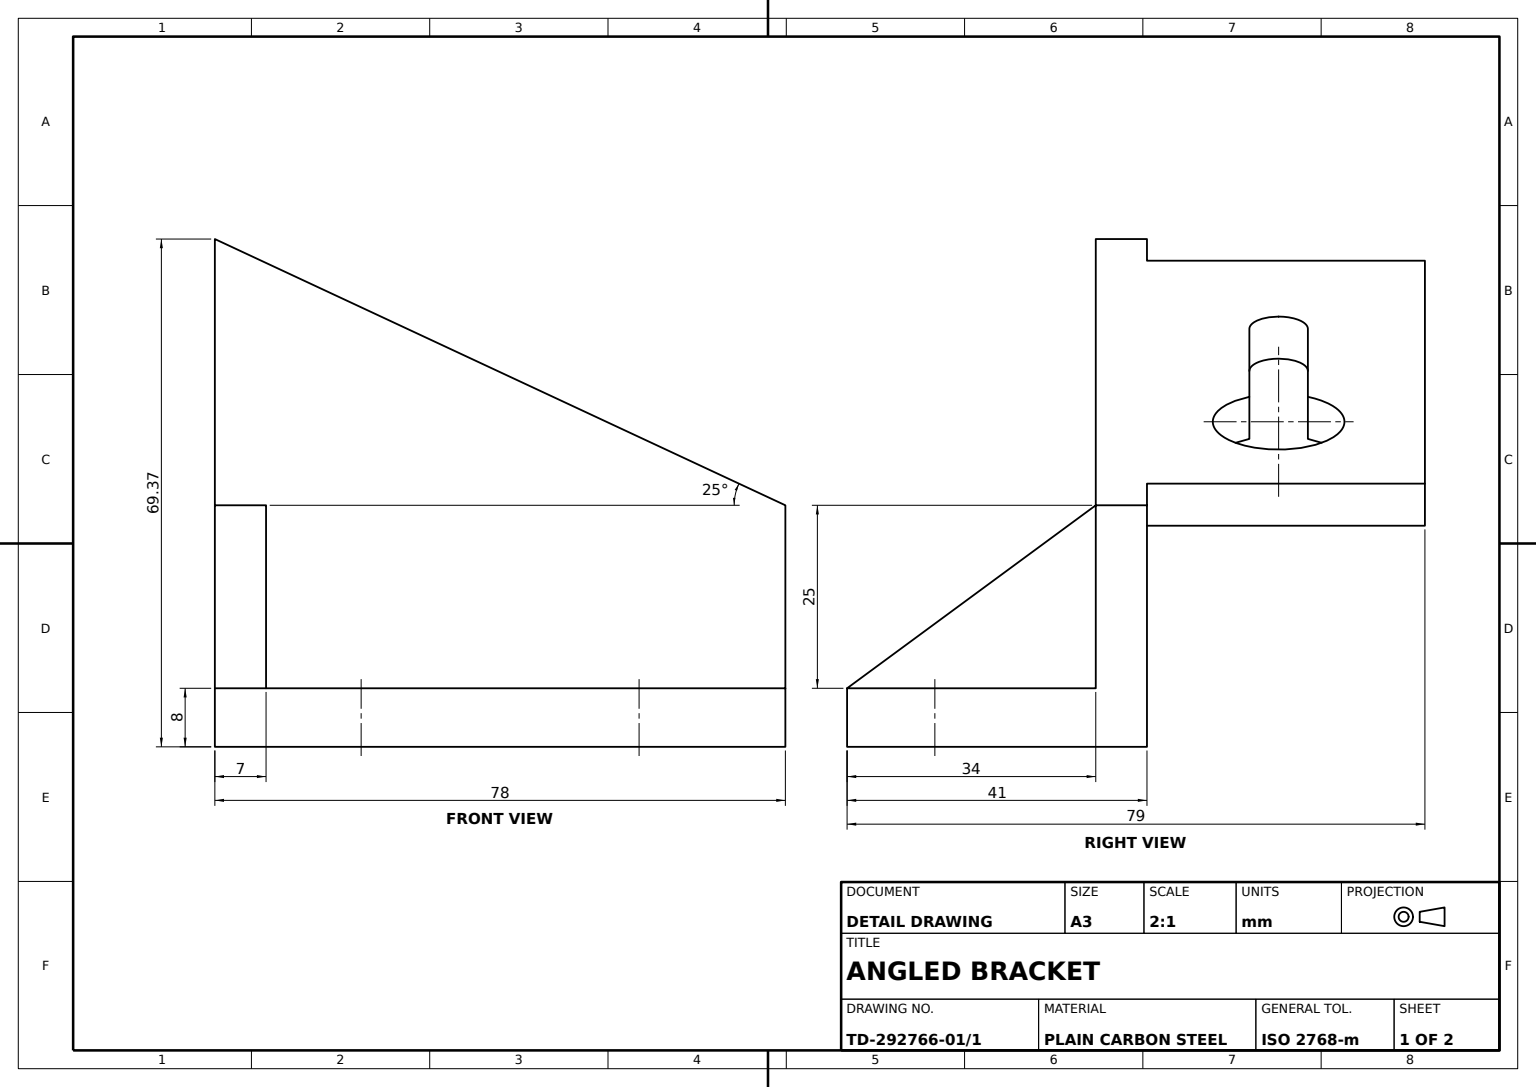
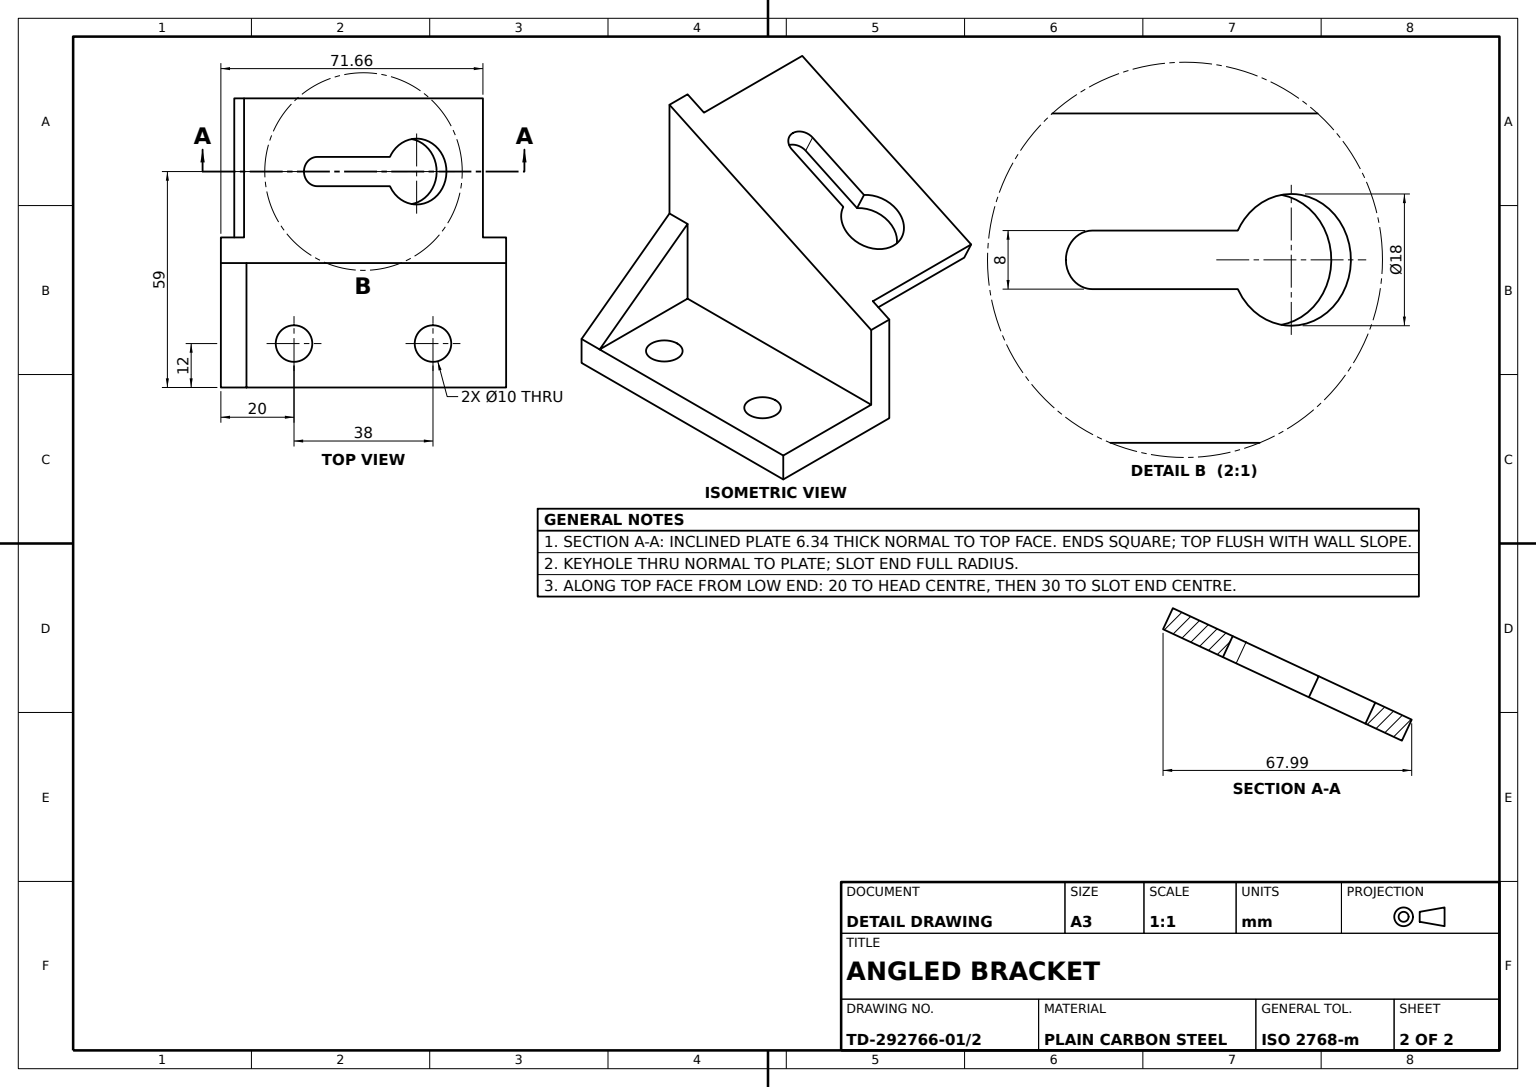
from build123d import *

# Parameters (mm, degrees)
BASE_PLATE_SKETCH_W                  = 78
BASE_PLATE_SKETCH_H                  = 41
BASE_PLATE_SKETCH_R                  = 5
BASE_PLATE_WITH_MOUNTING_HOLES_DEPTH = 8
UPRIGHT_WALL_SKETCH_W                = 7
UPRIGHT_WALL_SKETCH_H                = 41
UPRIGHT_WALL_DEPTH                   = 38
BACK_PLATE_SKETCH_W                  = 78
BACK_PLATE_SKETCH_H                  = 7
BACK_PLATE_DEPTH                     = 82
WALL_TRIM_CUT_DEPTH                  = 58
ANGLED_TRIM_CUT_25DEG_DEPTH          = 58
INCLINED_FLANGE_DEPTH                = 38
FLANGE_PROFILE_CUT_SKETCH_W          = 9.958327832
FLANGE_PROFILE_CUT_SKETCH_H          = 38
FLANGE_PROFILE_CUT_SKETCH_W_2        = 7
FLANGE_PROFILE_CUT_DEPTH             = 38
KEYHOLE_SLOT_DIA18_X_W8_REACH        = 92.402


with BuildPart() as part:
    # Base Plate Sketch → Base Plate with Mounting Holes (new body)
    with BuildSketch(Plane(origin=(0, 0, 0), x_dir=(1, 0, 0), z_dir=(0, 1, 0))):
        with Locations((0, -4)):
            Rectangle(BASE_PLATE_SKETCH_W, BASE_PLATE_SKETCH_H)
        with Locations(Location((-19, -12.5, 0), (0, 0, 270))):
            Circle(BASE_PLATE_SKETCH_R, mode=Mode.SUBTRACT)
        with Locations(Location((19, -12.5, 0), (0, 0, 270))):
            Circle(BASE_PLATE_SKETCH_R, mode=Mode.SUBTRACT)
    extrude(amount=BASE_PLATE_WITH_MOUNTING_HOLES_DEPTH)

    # Upright Wall Sketch → Upright Wall (add)
    with BuildSketch(Plane(origin=(0, 8, 0), x_dir=(1, 0, 0), z_dir=(0, 1, 0))):
        with Locations((-35.5, -4)):
            Rectangle(UPRIGHT_WALL_SKETCH_W, UPRIGHT_WALL_SKETCH_H)
    extrude(amount=UPRIGHT_WALL_DEPTH)

    # Back Plate Sketch → Back Plate (add)
    with BuildSketch(Plane(origin=(0, 8, 0), x_dir=(1, 0, 0), z_dir=(0, 1, 0))):
        with Locations((0, 13)):
            Rectangle(BACK_PLATE_SKETCH_W, BACK_PLATE_SKETCH_H)
    extrude(amount=BACK_PLATE_DEPTH)

    # Wall Trim Sketch → Wall Trim Cut (cut)
    with BuildSketch(Plane(origin=(-32, 0, 0), x_dir=(0, 0, -1), z_dir=(1, 0, 0))):
        Polygon((9.5, 33), (-24.5, 8), (-24.5, 46), (9.5, 46), align=None)
    extrude(amount=-WALL_TRIM_CUT_DEPTH, mode=Mode.SUBTRACT)

    # Angled Trim Sketch 25deg → Angled Trim Cut 25deg (cut)
    with BuildSketch(Plane.XY.offset(-9.5)):
        Polygon((-39, 69.371997336), (39, 33), (39, 90), (-39, 90), align=None)
    extrude(amount=-ANGLED_TRIM_CUT_25DEG_DEPTH, mode=Mode.SUBTRACT)

    # Inclined Flange Sketch → Inclined Flange (add)
    with BuildSketch(Plane(origin=(0, 0, -16.5), x_dir=(-1, 0, 0), z_dir=(0, 0, -1))):
        Polygon((-39, 33), (39, 69.371997336), (39, 62.371997336), (-39, 26), align=None)
    extrude(amount=INCLINED_FLANGE_DEPTH)

    # Flange Profile Cut Sketch → Flange Profile Cut (cut)
    with BuildSketch(Plane(origin=(19.605374923, 42.043862201, 0), x_dir=(0.9063077870366495, -0.42261826174070033, 0), z_dir=(0.42261826174070033, 0.9063077870366495, 0))):
        with Locations((19.378764973, 35.5)):
            Rectangle(FLANGE_PROFILE_CUT_SKETCH_W, FLANGE_PROFILE_CUT_SKETCH_H)
        with Locations((-61.163876622, 35.5)):
            Rectangle(FLANGE_PROFILE_CUT_SKETCH_W_2, FLANGE_PROFILE_CUT_SKETCH_H)
    extrude(amount=-FLANGE_PROFILE_CUT_DEPTH, mode=Mode.SUBTRACT)

    # Keyhole Slot Sketch → Keyhole Slot Dia18 x W8 (cut, up to next)
    with BuildSketch(Plane(origin=(19.605374923, 42.043862201, 0), x_dir=(0.9063077870366495, -0.42261826174070033, 0), z_dir=(0.42261826174070033, 0.9063077870366495, 0)), mode=Mode.PRIVATE) as keyhole_slot_dia18_x_w8_sk1:
        with BuildLine():
            Line((-35.600398943, 38.5), (-13.662656691, 38.5))
            ThreePointArc((-13.662656691, 38.5), (3.399601057, 34.5), (-13.662656691, 30.5))
            Line((-13.662656691, 30.5), (-35.600398943, 30.5))
            ThreePointArc((-35.600398943, 30.5), (-39.600398943, 34.5), (-35.600398943, 38.5))
        make_face()
    keyhole_slot_dia18_x_w8_tool1 = extrude(keyhole_slot_dia18_x_w8_sk1.sketch, amount=-KEYHOLE_SLOT_DIA18_X_W8_REACH, mode=Mode.PRIVATE) & part.part
    add(keyhole_slot_dia18_x_w8_tool1.solids().sort_by_distance((6.285215, 48.255155, -34.5))[0], mode=Mode.SUBTRACT)


solid = part.part
